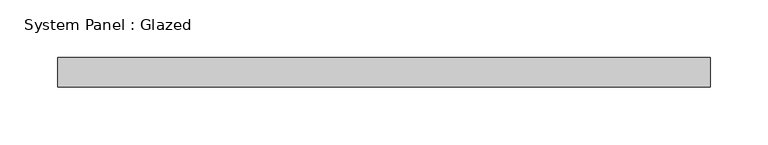
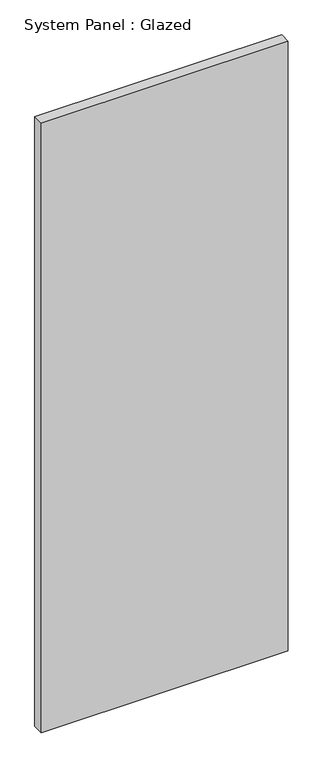
"""IFC4 building model written with IfcOpenShell, lengths in millimetres: plate geometry, System Panel : Glazed."""

from ifc_helpers import new_model, si_unit, origin, origin_with_axes, place, context, project, spatial, polyline, outline, extrude, source, transform, mapped, element, save


def system_panel_glazed_22e8721b(model_context):
    return source(origin(), model_context, "Body", "SweptSolid", [
        extrude(outline(polyline([(282.575, 19.05), (-282.575, 19.05), (-282.575, 44.45), (282.575, 44.45), (282.575, 19.05)])), origin_with_axes(), (0.0, 0.0, 1.0), 1474.4580508),
    ])


if __name__ == "__main__":
    model = new_model("IFC4")
    model_context = context("Model", 3, world=origin())
    ifc_project = project(units=[si_unit("LENGTHUNIT", "METRE", prefix="MILLI")], contexts=[model_context])
    site = spatial("IfcSite", under=ifc_project)
    building = spatial("IfcBuilding", under=site)
    placement = place(None, origin())
    system_panel_glazed_shape = system_panel_glazed_22e8721b(model_context)
    element("IfcPlate", 1, ObjectType="System Panel : Glazed", at=placement, inside=building, context=model_context, shape_type="MappedRepresentation", body=[
        mapped(system_panel_glazed_shape, transform((0.0, 0.0, 0.0), x_axis=(1.0, 0.0, 0.0), y_axis=(0.0, 1.0, 0.0), z_axis=(0.0, 0.0, 1.0))),
    ])
    save(model, "model.ifc")

# Revit data of these elements
# Type "System Panel : Glazed"
#   Construction Type Id = "GSP4R"
#   Analytic Construction = "1/8 in Pilkington single glazing"
#   Visual Light Transmittance = 0.9
#   Solar Heat Gain Coefficient = 0.86
#   Heat Transfer Coefficient (U) = 1.18115 BTU/(h·ft²·°F)
#   Define Thermal Properties by = 1
# Element 1 (IfcPlate, "System Panel : Glazed")
#   Materials on its faces: "Glass"
# Materials
#   "Glass": class "Glass", colour RGB 0 128 192, transparency 0.75, Description = "Soda Lime Glass", Cost = 0
